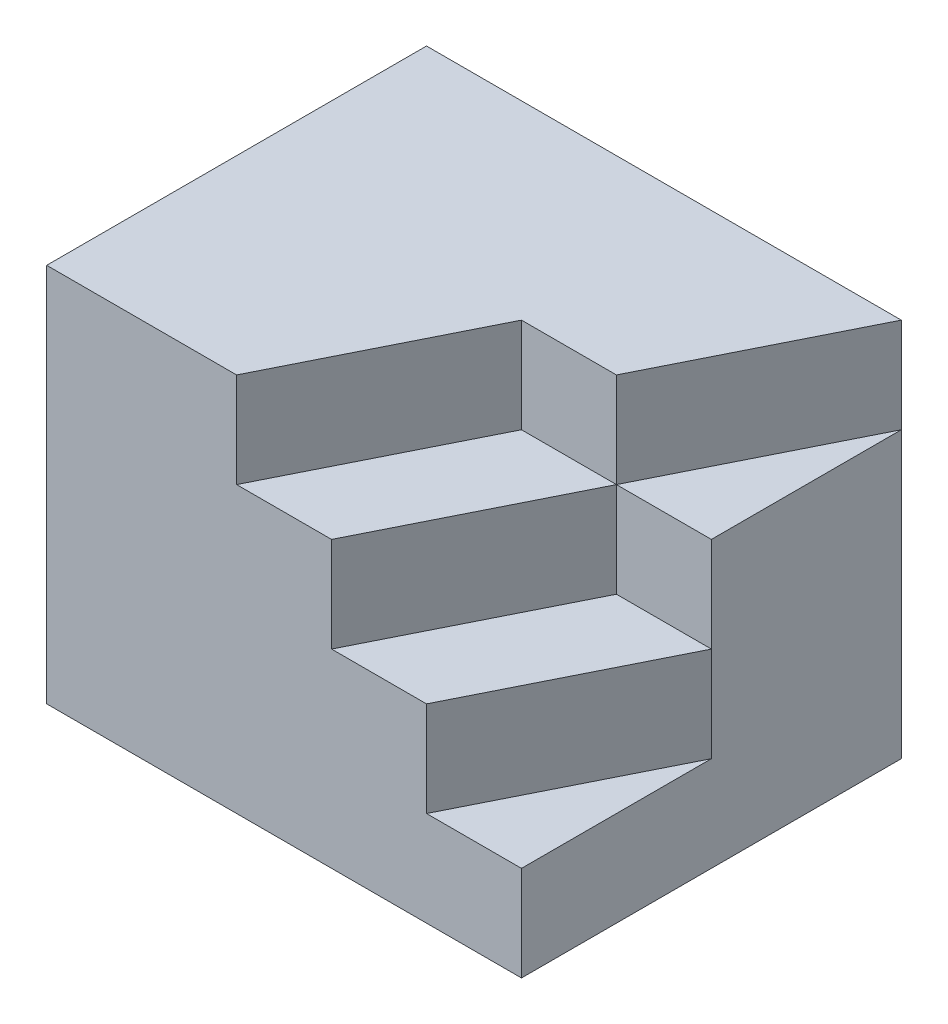
ISO-10303-21;
HEADER;
FILE_DESCRIPTION(('STEP AP214'),'2;1');
FILE_NAME('part.step','',(''),(''),'','','');
FILE_SCHEMA(('AUTOMOTIVE_DESIGN { 1 0 10303 214 1 1 1 1 }'));
ENDSEC;
DATA;
#1=APPLICATION_CONTEXT('core data for automotive mechanical design processes');
#2=APPLICATION_PROTOCOL_DEFINITION('international standard','automotive_design',2000,#1);
#3=PRODUCT_CONTEXT('',#1,'mechanical');
#4=PRODUCT('Part','Part','',(#3));
#5=PRODUCT_RELATED_PRODUCT_CATEGORY('part','',(#4));
#6=PRODUCT_DEFINITION_FORMATION('','',#4);
#7=PRODUCT_DEFINITION_CONTEXT('part definition',#1,'design');
#8=PRODUCT_DEFINITION('design','',#6,#7);
#9=PRODUCT_DEFINITION_SHAPE('','',#8);
#10=(LENGTH_UNIT() NAMED_UNIT(*) SI_UNIT(.MILLI.,.METRE.));
#11=(NAMED_UNIT(*) PLANE_ANGLE_UNIT() SI_UNIT($,.RADIAN.));
#12=(NAMED_UNIT(*) SI_UNIT($,.STERADIAN.) SOLID_ANGLE_UNIT());
#13=UNCERTAINTY_MEASURE_WITH_UNIT(LENGTH_MEASURE(1.E-05),#10,'distance_accuracy_value','');
#14=(GEOMETRIC_REPRESENTATION_CONTEXT(3) GLOBAL_UNCERTAINTY_ASSIGNED_CONTEXT((#13)) GLOBAL_UNIT_ASSIGNED_CONTEXT((#10,
#11,#12)) REPRESENTATION_CONTEXT('',''));
#15=CARTESIAN_POINT('',(0.,0.,0.));
#16=DIRECTION('',(0.,0.,1.));
#17=DIRECTION('',(1.,0.,0.));
#18=AXIS2_PLACEMENT_3D('',#15,#16,#17);
#19=CARTESIAN_POINT('',(25.,20.,20.));
#20=DIRECTION('',(-1.,0.,0.));
#21=DIRECTION('',(0.,0.,1.));
#22=AXIS2_PLACEMENT_3D('',#19,#20,#21);
#23=PLANE('',#22);
#24=DIRECTION('',(0.,1.,0.));
#25=VECTOR('',#24,1.);
#26=CARTESIAN_POINT('',(25.,0.,0.));
#27=LINE('',#26,#25);
#28=CARTESIAN_POINT('',(25.,0.,0.));
#29=VERTEX_POINT('',#28);
#30=CARTESIAN_POINT('',(25.,10.,0.));
#31=VERTEX_POINT('',#30);
#32=EDGE_CURVE('E160',#29,#31,#27,.T.);
#33=ORIENTED_EDGE('',*,*,#32,.F.);
#34=DIRECTION('',(0.,1.,0.));
#35=VECTOR('',#34,1.);
#36=CARTESIAN_POINT('',(25.,-10.,0.));
#37=LINE('',#36,#35);
#38=CARTESIAN_POINT('',(25.,-10.,0.));
#39=VERTEX_POINT('',#38);
#40=EDGE_CURVE('E139',#39,#29,#37,.T.);
#41=ORIENTED_EDGE('',*,*,#40,.F.);
#42=DIRECTION('',(0.,0.,-1.));
#43=VECTOR('',#42,1.);
#44=CARTESIAN_POINT('',(25.,-10.,0.));
#45=LINE('',#44,#43);
#46=CARTESIAN_POINT('',(25.,-10.,20.));
#47=VERTEX_POINT('',#46);
#48=EDGE_CURVE('E150',#47,#39,#45,.T.);
#49=ORIENTED_EDGE('',*,*,#48,.F.);
#50=DIRECTION('',(0.,-1.,0.));
#51=VECTOR('',#50,1.);
#52=CARTESIAN_POINT('',(25.,20.,20.));
#53=LINE('',#52,#51);
#54=CARTESIAN_POINT('',(25.,-20.,20.));
#55=VERTEX_POINT('',#54);
#56=EDGE_CURVE('E49',#47,#55,#53,.T.);
#57=ORIENTED_EDGE('',*,*,#56,.T.);
#58=DIRECTION('',(0.,0.,-1.));
#59=VECTOR('',#58,1.);
#60=CARTESIAN_POINT('',(25.,-20.,20.));
#61=LINE('',#60,#59);
#62=CARTESIAN_POINT('',(25.,-20.,-20.));
#63=VERTEX_POINT('',#62);
#64=EDGE_CURVE('E224',#55,#63,#61,.T.);
#65=ORIENTED_EDGE('',*,*,#64,.T.);
#66=DIRECTION('',(0.,-1.,0.));
#67=VECTOR('',#66,1.);
#68=CARTESIAN_POINT('',(25.,20.,-20.));
#69=LINE('',#68,#67);
#70=CARTESIAN_POINT('',(25.,10.,-20.));
#71=VERTEX_POINT('',#70);
#72=EDGE_CURVE('E77',#71,#63,#69,.T.);
#73=ORIENTED_EDGE('',*,*,#72,.F.);
#74=DIRECTION('',(0.,0.,-1.));
#75=VECTOR('',#74,1.);
#76=CARTESIAN_POINT('',(25.,10.,0.));
#77=LINE('',#76,#75);
#78=EDGE_CURVE('E183',#31,#71,#77,.T.);
#79=ORIENTED_EDGE('',*,*,#78,.F.);
#80=EDGE_LOOP('',(#33,#41,#49,#57,#65,#73,#79));
#81=FACE_BOUND('',#80,.T.);
#82=ADVANCED_FACE('F41',(#81),#23,.F.);
#83=CARTESIAN_POINT('',(0.,10.,0.));
#84=DIRECTION('',(0.,1.,0.));
#85=DIRECTION('',(0.,0.,1.));
#86=AXIS2_PLACEMENT_3D('',#83,#84,#85);
#87=PLANE('',#86);
#88=DIRECTION('',(-0.447213595499958,0.,0.894427190999916));
#89=VECTOR('',#88,1.);
#90=CARTESIAN_POINT('',(12.,10.,6.));
#91=LINE('',#90,#89);
#92=CARTESIAN_POINT('',(15.,10.,0.));
#93=VERTEX_POINT('',#92);
#94=EDGE_CURVE('E187',#71,#93,#91,.T.);
#95=ORIENTED_EDGE('',*,*,#94,.T.);
#96=DIRECTION('',(1.,0.,0.));
#97=VECTOR('',#96,1.);
#98=CARTESIAN_POINT('',(0.,10.,0.));
#99=LINE('',#98,#97);
#100=EDGE_CURVE('E157',#93,#31,#99,.T.);
#101=ORIENTED_EDGE('',*,*,#100,.T.);
#102=ORIENTED_EDGE('',*,*,#78,.T.);
#103=EDGE_LOOP('',(#95,#101,#102));
#104=FACE_BOUND('',#103,.T.);
#105=ADVANCED_FACE('F253',(#104),#87,.T.);
#106=CARTESIAN_POINT('',(-25.,20.,20.));
#107=DIRECTION('',(1.,0.,0.));
#108=DIRECTION('',(0.,0.,-1.));
#109=AXIS2_PLACEMENT_3D('',#106,#107,#108);
#110=PLANE('',#109);
#111=DIRECTION('',(0.,0.,1.));
#112=VECTOR('',#111,1.);
#113=CARTESIAN_POINT('',(-25.,-20.,20.));
#114=LINE('',#113,#112);
#115=CARTESIAN_POINT('',(-25.,-20.,-20.));
#116=VERTEX_POINT('',#115);
#117=CARTESIAN_POINT('',(-25.,-20.,20.));
#118=VERTEX_POINT('',#117);
#119=EDGE_CURVE('E207',#116,#118,#114,.T.);
#120=ORIENTED_EDGE('',*,*,#119,.T.);
#121=DIRECTION('',(0.,-1.,0.));
#122=VECTOR('',#121,1.);
#123=CARTESIAN_POINT('',(-25.,20.,20.));
#124=LINE('',#123,#122);
#125=CARTESIAN_POINT('',(-25.,20.,20.));
#126=VERTEX_POINT('',#125);
#127=EDGE_CURVE('E12',#126,#118,#124,.T.);
#128=ORIENTED_EDGE('',*,*,#127,.F.);
#129=DIRECTION('',(0.,0.,1.));
#130=VECTOR('',#129,1.);
#131=CARTESIAN_POINT('',(-25.,20.,20.));
#132=LINE('',#131,#130);
#133=CARTESIAN_POINT('',(-25.,20.,-20.));
#134=VERTEX_POINT('',#133);
#135=EDGE_CURVE('E213',#134,#126,#132,.T.);
#136=ORIENTED_EDGE('',*,*,#135,.F.);
#137=DIRECTION('',(0.,-1.,0.));
#138=VECTOR('',#137,1.);
#139=CARTESIAN_POINT('',(-25.,20.,-20.));
#140=LINE('',#139,#138);
#141=EDGE_CURVE('E220',#134,#116,#140,.T.);
#142=ORIENTED_EDGE('',*,*,#141,.T.);
#143=EDGE_LOOP('',(#120,#128,#136,#142));
#144=FACE_BOUND('',#143,.T.);
#145=ADVANCED_FACE('F43',(#144),#110,.F.);
#146=CARTESIAN_POINT('',(25.,20.,20.));
#147=DIRECTION('',(0.,0.,-1.));
#148=DIRECTION('',(-1.,0.,0.));
#149=AXIS2_PLACEMENT_3D('',#146,#147,#148);
#150=PLANE('',#149);
#151=DIRECTION('',(1.,0.,0.));
#152=VECTOR('',#151,1.);
#153=CARTESIAN_POINT('',(0.,-10.,20.));
#154=LINE('',#153,#152);
#155=CARTESIAN_POINT('',(15.,-10.,20.));
#156=VERTEX_POINT('',#155);
#157=EDGE_CURVE('E148',#156,#47,#154,.T.);
#158=ORIENTED_EDGE('',*,*,#157,.F.);
#159=DIRECTION('',(0.,1.,0.));
#160=VECTOR('',#159,1.);
#161=CARTESIAN_POINT('',(15.,-10.,20.));
#162=LINE('',#161,#160);
#163=CARTESIAN_POINT('',(15.,0.,20.));
#164=VERTEX_POINT('',#163);
#165=EDGE_CURVE('E141',#156,#164,#162,.T.);
#166=ORIENTED_EDGE('',*,*,#165,.T.);
#167=DIRECTION('',(1.,0.,0.));
#168=VECTOR('',#167,1.);
#169=CARTESIAN_POINT('',(0.,0.,20.));
#170=LINE('',#169,#168);
#171=CARTESIAN_POINT('',(4.99999999999999,0.,20.));
#172=VERTEX_POINT('',#171);
#173=EDGE_CURVE('E171',#172,#164,#170,.T.);
#174=ORIENTED_EDGE('',*,*,#173,.F.);
#175=DIRECTION('',(0.,1.,0.));
#176=VECTOR('',#175,1.);
#177=CARTESIAN_POINT('',(4.99999999999999,0.,20.));
#178=LINE('',#177,#176);
#179=CARTESIAN_POINT('',(4.99999999999999,10.,20.));
#180=VERTEX_POINT('',#179);
#181=EDGE_CURVE('E179',#172,#180,#178,.T.);
#182=ORIENTED_EDGE('',*,*,#181,.T.);
#183=DIRECTION('',(1.,0.,0.));
#184=VECTOR('',#183,1.);
#185=CARTESIAN_POINT('',(0.,10.,20.));
#186=LINE('',#185,#184);
#187=CARTESIAN_POINT('',(-5.,10.,20.));
#188=VERTEX_POINT('',#187);
#189=EDGE_CURVE('E197',#188,#180,#186,.T.);
#190=ORIENTED_EDGE('',*,*,#189,.F.);
#191=DIRECTION('',(0.,1.,0.));
#192=VECTOR('',#191,1.);
#193=CARTESIAN_POINT('',(-5.,10.,20.));
#194=LINE('',#193,#192);
#195=CARTESIAN_POINT('',(-5.,20.,20.));
#196=VERTEX_POINT('',#195);
#197=EDGE_CURVE('E210',#188,#196,#194,.T.);
#198=ORIENTED_EDGE('',*,*,#197,.T.);
#199=DIRECTION('',(1.,0.,0.));
#200=VECTOR('',#199,1.);
#201=CARTESIAN_POINT('',(25.,20.,20.));
#202=LINE('',#201,#200);
#203=EDGE_CURVE('E88',#126,#196,#202,.T.);
#204=ORIENTED_EDGE('',*,*,#203,.F.);
#205=ORIENTED_EDGE('',*,*,#127,.T.);
#206=DIRECTION('',(1.,0.,0.));
#207=VECTOR('',#206,1.);
#208=CARTESIAN_POINT('',(25.,-20.,20.));
#209=LINE('',#208,#207);
#210=EDGE_CURVE('E219',#118,#55,#209,.T.);
#211=ORIENTED_EDGE('',*,*,#210,.T.);
#212=ORIENTED_EDGE('',*,*,#56,.F.);
#213=EDGE_LOOP('',(#158,#166,#174,#182,#190,#198,#204,#205,#211,#212));
#214=FACE_BOUND('',#213,.T.);
#215=ADVANCED_FACE('F228',(#214),#150,.F.);
#216=CARTESIAN_POINT('',(25.,20.,-20.));
#217=DIRECTION('',(0.,0.,1.));
#218=DIRECTION('',(1.,0.,0.));
#219=AXIS2_PLACEMENT_3D('',#216,#217,#218);
#220=PLANE('',#219);
#221=DIRECTION('',(-1.,0.,0.));
#222=VECTOR('',#221,1.);
#223=CARTESIAN_POINT('',(25.,-20.,-20.));
#224=LINE('',#223,#222);
#225=EDGE_CURVE('E80',#63,#116,#224,.T.);
#226=ORIENTED_EDGE('',*,*,#225,.T.);
#227=ORIENTED_EDGE('',*,*,#141,.F.);
#228=DIRECTION('',(-1.,0.,0.));
#229=VECTOR('',#228,1.);
#230=CARTESIAN_POINT('',(25.,20.,-20.));
#231=LINE('',#230,#229);
#232=CARTESIAN_POINT('',(25.,20.,-20.));
#233=VERTEX_POINT('',#232);
#234=EDGE_CURVE('E59',#233,#134,#231,.T.);
#235=ORIENTED_EDGE('',*,*,#234,.F.);
#236=EDGE_CURVE('E227',#233,#71,#69,.T.);
#237=ORIENTED_EDGE('',*,*,#236,.T.);
#238=ORIENTED_EDGE('',*,*,#72,.T.);
#239=EDGE_LOOP('',(#226,#227,#235,#237,#238));
#240=FACE_BOUND('',#239,.T.);
#241=ADVANCED_FACE('F237',(#240),#220,.F.);
#242=CARTESIAN_POINT('',(0.,20.,0.));
#243=DIRECTION('',(0.,1.,0.));
#244=DIRECTION('',(0.,0.,1.));
#245=AXIS2_PLACEMENT_3D('',#242,#243,#244);
#246=PLANE('',#245);
#247=DIRECTION('',(-0.447213595499958,0.,0.894427190999916));
#248=VECTOR('',#247,1.);
#249=CARTESIAN_POINT('',(4.,20.,2.));
#250=LINE('',#249,#248);
#251=CARTESIAN_POINT('',(5.,20.,0.));
#252=VERTEX_POINT('',#251);
#253=EDGE_CURVE('E189',#252,#196,#250,.T.);
#254=ORIENTED_EDGE('',*,*,#253,.F.);
#255=DIRECTION('',(-1.,0.,0.));
#256=VECTOR('',#255,1.);
#257=CARTESIAN_POINT('',(0.,20.,0.));
#258=LINE('',#257,#256);
#259=CARTESIAN_POINT('',(15.,20.,0.));
#260=VERTEX_POINT('',#259);
#261=EDGE_CURVE('E201',#260,#252,#258,.T.);
#262=ORIENTED_EDGE('',*,*,#261,.F.);
#263=DIRECTION('',(-0.447213595499958,0.,0.894427190999916));
#264=VECTOR('',#263,1.);
#265=CARTESIAN_POINT('',(12.,20.,6.));
#266=LINE('',#265,#264);
#267=EDGE_CURVE('E177',#233,#260,#266,.T.);
#268=ORIENTED_EDGE('',*,*,#267,.F.);
#269=ORIENTED_EDGE('',*,*,#234,.T.);
#270=ORIENTED_EDGE('',*,*,#135,.T.);
#271=ORIENTED_EDGE('',*,*,#203,.T.);
#272=EDGE_LOOP('',(#254,#262,#268,#269,#270,#271));
#273=FACE_BOUND('',#272,.T.);
#274=ADVANCED_FACE('F244',(#273),#246,.T.);
#275=CARTESIAN_POINT('',(0.,-20.,0.));
#276=DIRECTION('',(0.,1.,0.));
#277=DIRECTION('',(0.,0.,1.));
#278=AXIS2_PLACEMENT_3D('',#275,#276,#277);
#279=PLANE('',#278);
#280=ORIENTED_EDGE('',*,*,#119,.F.);
#281=ORIENTED_EDGE('',*,*,#225,.F.);
#282=ORIENTED_EDGE('',*,*,#64,.F.);
#283=ORIENTED_EDGE('',*,*,#210,.F.);
#284=EDGE_LOOP('',(#280,#281,#282,#283));
#285=FACE_BOUND('',#284,.T.);
#286=ADVANCED_FACE('F233',(#285),#279,.F.);
#287=CARTESIAN_POINT('',(4.,10.,2.));
#288=DIRECTION('',(-0.894427190999916,0.,-0.447213595499958));
#289=DIRECTION('',(-0.447213595499958,0.,0.894427190999916));
#290=AXIS2_PLACEMENT_3D('',#287,#288,#289);
#291=PLANE('',#290);
#292=ORIENTED_EDGE('',*,*,#253,.T.);
#293=ORIENTED_EDGE('',*,*,#197,.F.);
#294=DIRECTION('',(-0.447213595499958,0.,0.894427190999916));
#295=VECTOR('',#294,1.);
#296=CARTESIAN_POINT('',(4.,10.,2.));
#297=LINE('',#296,#295);
#298=CARTESIAN_POINT('',(5.,10.,0.));
#299=VERTEX_POINT('',#298);
#300=EDGE_CURVE('E192',#299,#188,#297,.T.);
#301=ORIENTED_EDGE('',*,*,#300,.F.);
#302=DIRECTION('',(0.,1.,0.));
#303=VECTOR('',#302,1.);
#304=CARTESIAN_POINT('',(5.,10.,0.));
#305=LINE('',#304,#303);
#306=EDGE_CURVE('E209',#299,#252,#305,.T.);
#307=ORIENTED_EDGE('',*,*,#306,.T.);
#308=EDGE_LOOP('',(#292,#293,#301,#307));
#309=FACE_BOUND('',#308,.T.);
#310=ADVANCED_FACE('F291',(#309),#291,.F.);
#311=CARTESIAN_POINT('',(0.,10.,0.));
#312=DIRECTION('',(0.,0.,-1.));
#313=DIRECTION('',(-1.,0.,0.));
#314=AXIS2_PLACEMENT_3D('',#311,#312,#313);
#315=PLANE('',#314);
#316=ORIENTED_EDGE('',*,*,#261,.T.);
#317=ORIENTED_EDGE('',*,*,#306,.F.);
#318=DIRECTION('',(-1.,0.,0.));
#319=VECTOR('',#318,1.);
#320=CARTESIAN_POINT('',(0.,10.,0.));
#321=LINE('',#320,#319);
#322=EDGE_CURVE('E191',#93,#299,#321,.T.);
#323=ORIENTED_EDGE('',*,*,#322,.F.);
#324=DIRECTION('',(0.,1.,0.));
#325=VECTOR('',#324,1.);
#326=CARTESIAN_POINT('',(15.,10.,0.));
#327=LINE('',#326,#325);
#328=EDGE_CURVE('E199',#93,#260,#327,.T.);
#329=ORIENTED_EDGE('',*,*,#328,.T.);
#330=EDGE_LOOP('',(#316,#317,#323,#329));
#331=FACE_BOUND('',#330,.T.);
#332=ADVANCED_FACE('F245',(#331),#315,.F.);
#333=CARTESIAN_POINT('',(12.,10.,6.));
#334=DIRECTION('',(-0.894427190999916,0.,-0.447213595499958));
#335=DIRECTION('',(-0.447213595499958,0.,0.894427190999916));
#336=AXIS2_PLACEMENT_3D('',#333,#334,#335);
#337=PLANE('',#336);
#338=ORIENTED_EDGE('',*,*,#267,.T.);
#339=ORIENTED_EDGE('',*,*,#328,.F.);
#340=ORIENTED_EDGE('',*,*,#94,.F.);
#341=ORIENTED_EDGE('',*,*,#236,.F.);
#342=EDGE_LOOP('',(#338,#339,#340,#341));
#343=FACE_BOUND('',#342,.T.);
#344=ADVANCED_FACE('F239',(#343),#337,.F.);
#345=DIRECTION('',(-0.447213595499958,0.,0.894427190999916));
#346=VECTOR('',#345,1.);
#347=CARTESIAN_POINT('',(12.,10.,6.));
#348=LINE('',#347,#346);
#349=EDGE_CURVE('E169',#93,#180,#348,.T.);
#350=ORIENTED_EDGE('',*,*,#349,.F.);
#351=ORIENTED_EDGE('',*,*,#322,.T.);
#352=ORIENTED_EDGE('',*,*,#300,.T.);
#353=ORIENTED_EDGE('',*,*,#189,.T.);
#354=EDGE_LOOP('',(#350,#351,#352,#353));
#355=FACE_BOUND('',#354,.T.);
#356=ADVANCED_FACE('F256',(#355),#87,.T.);
#357=CARTESIAN_POINT('',(0.,0.,0.));
#358=DIRECTION('',(0.,0.,1.));
#359=DIRECTION('',(1.,0.,0.));
#360=AXIS2_PLACEMENT_3D('',#357,#358,#359);
#361=PLANE('',#360);
#362=ORIENTED_EDGE('',*,*,#100,.F.);
#363=DIRECTION('',(0.,1.,0.));
#364=VECTOR('',#363,1.);
#365=CARTESIAN_POINT('',(15.,0.,0.));
#366=LINE('',#365,#364);
#367=CARTESIAN_POINT('',(15.,0.,0.));
#368=VERTEX_POINT('',#367);
#369=EDGE_CURVE('E173',#368,#93,#366,.T.);
#370=ORIENTED_EDGE('',*,*,#369,.F.);
#371=DIRECTION('',(1.,0.,0.));
#372=VECTOR('',#371,1.);
#373=CARTESIAN_POINT('',(0.,0.,0.));
#374=LINE('',#373,#372);
#375=EDGE_CURVE('E163',#368,#29,#374,.T.);
#376=ORIENTED_EDGE('',*,*,#375,.T.);
#377=ORIENTED_EDGE('',*,*,#32,.T.);
#378=EDGE_LOOP('',(#362,#370,#376,#377));
#379=FACE_BOUND('',#378,.T.);
#380=ADVANCED_FACE('F251',(#379),#361,.T.);
#381=CARTESIAN_POINT('',(12.,0.,6.));
#382=DIRECTION('',(-0.894427190999916,0.,-0.447213595499958));
#383=DIRECTION('',(-0.447213595499958,0.,0.894427190999916));
#384=AXIS2_PLACEMENT_3D('',#381,#382,#383);
#385=PLANE('',#384);
#386=ORIENTED_EDGE('',*,*,#349,.T.);
#387=ORIENTED_EDGE('',*,*,#181,.F.);
#388=DIRECTION('',(-0.447213595499958,0.,0.894427190999916));
#389=VECTOR('',#388,1.);
#390=CARTESIAN_POINT('',(12.,0.,6.));
#391=LINE('',#390,#389);
#392=EDGE_CURVE('E170',#368,#172,#391,.T.);
#393=ORIENTED_EDGE('',*,*,#392,.F.);
#394=ORIENTED_EDGE('',*,*,#369,.T.);
#395=EDGE_LOOP('',(#386,#387,#393,#394));
#396=FACE_BOUND('',#395,.T.);
#397=ADVANCED_FACE('F260',(#396),#385,.F.);
#398=CARTESIAN_POINT('',(0.,0.,0.));
#399=DIRECTION('',(0.,1.,0.));
#400=DIRECTION('',(0.,0.,1.));
#401=AXIS2_PLACEMENT_3D('',#398,#399,#400);
#402=PLANE('',#401);
#403=DIRECTION('',(-0.447213595499958,0.,0.894427190999916));
#404=VECTOR('',#403,1.);
#405=CARTESIAN_POINT('',(20.,0.,10.));
#406=LINE('',#405,#404);
#407=EDGE_CURVE('E153',#29,#164,#406,.T.);
#408=ORIENTED_EDGE('',*,*,#407,.F.);
#409=ORIENTED_EDGE('',*,*,#375,.F.);
#410=ORIENTED_EDGE('',*,*,#392,.T.);
#411=ORIENTED_EDGE('',*,*,#173,.T.);
#412=EDGE_LOOP('',(#408,#409,#410,#411));
#413=FACE_BOUND('',#412,.T.);
#414=ADVANCED_FACE('F265',(#413),#402,.T.);
#415=CARTESIAN_POINT('',(20.,-10.,10.));
#416=DIRECTION('',(-0.894427190999916,0.,-0.447213595499958));
#417=DIRECTION('',(-0.447213595499958,0.,0.894427190999916));
#418=AXIS2_PLACEMENT_3D('',#415,#416,#417);
#419=PLANE('',#418);
#420=ORIENTED_EDGE('',*,*,#407,.T.);
#421=ORIENTED_EDGE('',*,*,#165,.F.);
#422=DIRECTION('',(-0.447213595499958,0.,0.894427190999916));
#423=VECTOR('',#422,1.);
#424=CARTESIAN_POINT('',(20.,-10.,10.));
#425=LINE('',#424,#423);
#426=EDGE_CURVE('E136',#39,#156,#425,.T.);
#427=ORIENTED_EDGE('',*,*,#426,.F.);
#428=ORIENTED_EDGE('',*,*,#40,.T.);
#429=EDGE_LOOP('',(#420,#421,#427,#428));
#430=FACE_BOUND('',#429,.T.);
#431=ADVANCED_FACE('F138',(#430),#419,.F.);
#432=CARTESIAN_POINT('',(0.,-10.,0.));
#433=DIRECTION('',(0.,1.,0.));
#434=DIRECTION('',(0.,0.,1.));
#435=AXIS2_PLACEMENT_3D('',#432,#433,#434);
#436=PLANE('',#435);
#437=ORIENTED_EDGE('',*,*,#48,.T.);
#438=ORIENTED_EDGE('',*,*,#426,.T.);
#439=ORIENTED_EDGE('',*,*,#157,.T.);
#440=EDGE_LOOP('',(#437,#438,#439));
#441=FACE_BOUND('',#440,.T.);
#442=ADVANCED_FACE('F147',(#441),#436,.T.);
#443=CLOSED_SHELL('',(#82,#105,#145,#215,#241,#274,#286,#310,#332,#344,#356,#380,#397,#414,#431,#442));
#444=MANIFOLD_SOLID_BREP('B2',#443);
#445=ADVANCED_BREP_SHAPE_REPRESENTATION('',(#18,#444),#14);
#446=SHAPE_DEFINITION_REPRESENTATION(#9,#445);
ENDSEC;
END-ISO-10303-21;
